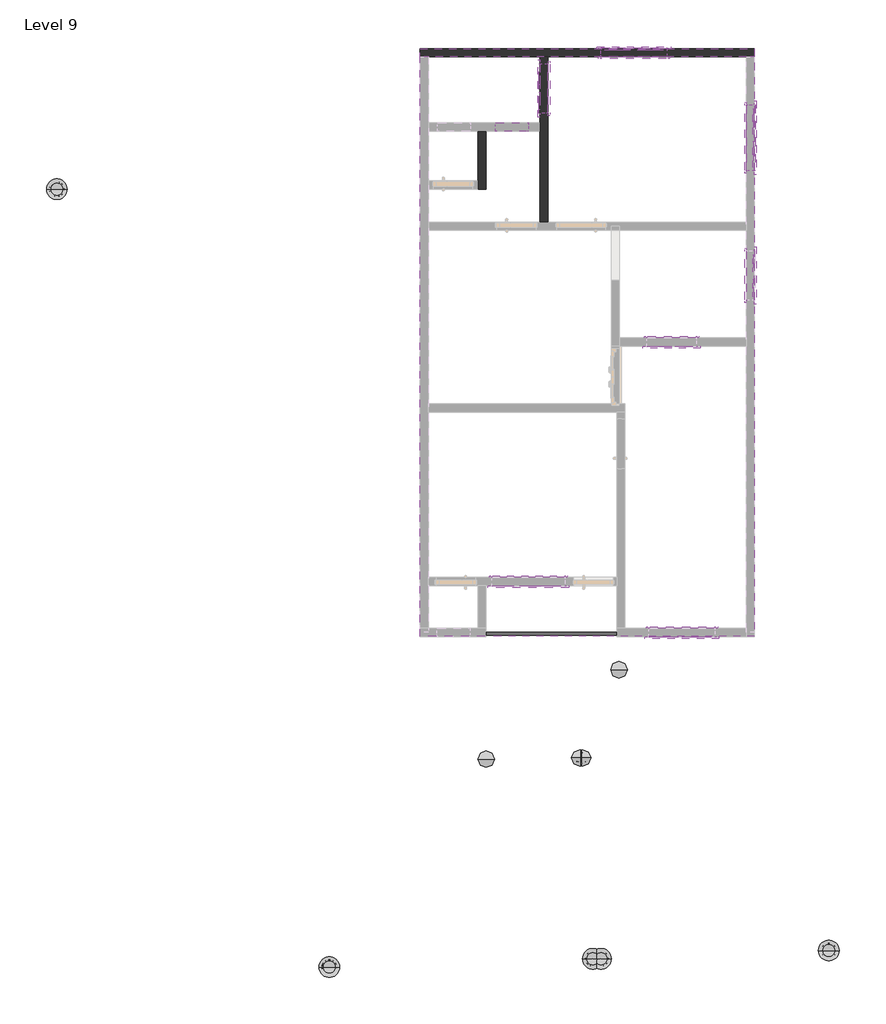
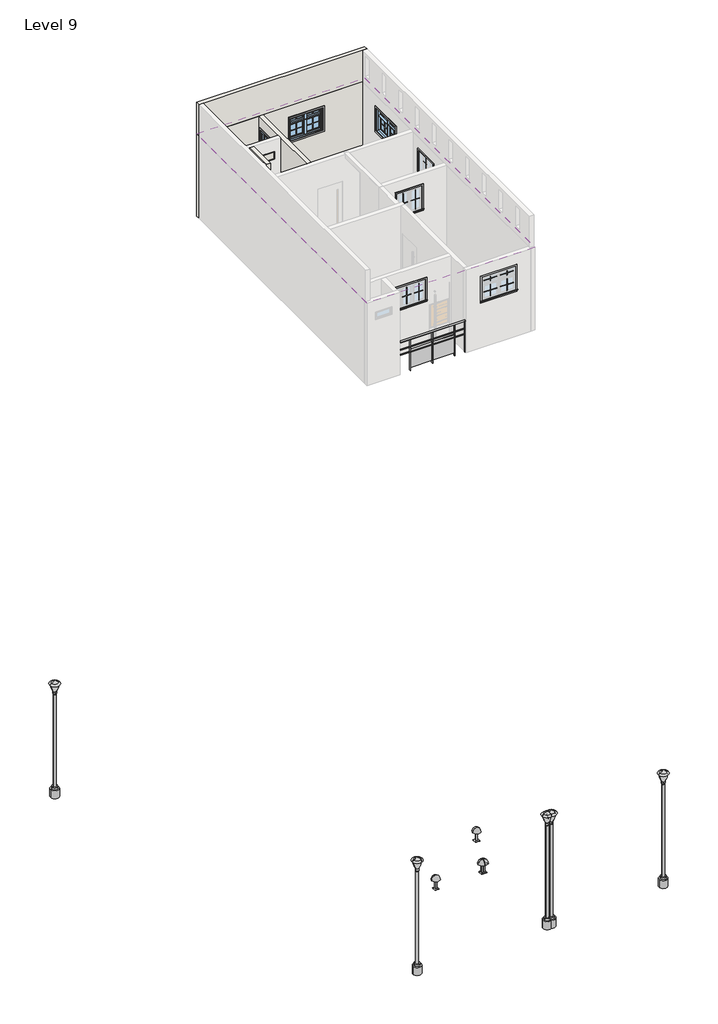
# One storey, part 2 of 2: 48 proxies, 10 light fixtures, 7 walls, 5 windows, 1 covering, 1 railing.
# Revit data of these elements (continued)
# Element 54 (IfcLightFixture, "M_Street Light - Antique : 400W Halogen - 120V")
#   Mark = "28"
#   Phase Created = New Construction
#   Materials on its faces: "Steel, Paint Finish, Dark Gray, Matte", "Glass, Frosted"
# Element 55 (IfcLightFixture, "M_Table Lamp - Hemispheric : 60W - 120V")
#   Mark = "8"
#   Phase Created = New Construction
#   Materials on its faces: "Steel, Chrome Plated", "Birch", "Plastic, Lamp Shade"
# Element 56 (IfcLightFixture, "M_Table Lamp - Hemispheric : 60W - 120V")
#   Mark = "9"
#   Phase Created = New Construction
#   Materials on its faces: "Steel, Chrome Plated", "Birch", "Plastic, Lamp Shade"
# Element 57 (IfcLightFixture, "M_Table Lamp - Hemispheric : 60W - 120V")
#   Mark = "10"
#   Phase Created = New Construction
#   Materials on its faces: "Steel, Chrome Plated", "Birch", "Plastic, Lamp Shade"
# Element 58 (IfcLightFixture, "M_Table Lamp - Hemispheric : 60W - 120V")
#   Mark = "11"
#   Phase Created = New Construction
#   Materials on its faces: "Steel, Chrome Plated", "Birch", "Plastic, Lamp Shade"
# Element 59 (IfcLightFixture, "M_Table Lamp - Hemispheric : 60W - 120V")
#   Mark = "13"
#   Phase Created = New Construction
#   Materials on its faces: "Steel, Chrome Plated", "Birch", "Plastic, Lamp Shade"
# Element 60 (IfcRailing, "Glass Panel - Bottom Fill")
#   Phase Created = New Construction
#   Materials on its faces: "Glass"
# Element 61 (IfcWall, "Generic - 6\"")
#   Top Offset = 0' - 0"
#   Base Offset = 0' - 0"
#   Unconnected Height = 10' - 6"
#   wall height = 10' - 6"
#   Phase Created = New Construction
#   Base Constraint = Level 9
#   Materials on its faces: "Default Wall", "Parking Stripe"
# Elements 62, 63, 64, 65, 66 (IfcWall, "Generic - 6\"")
#   Top Offset = 0' - 0"
#   Base Offset = 0' - 0"
#   Unconnected Height = 10' - 6"
#   wall height = 10' - 6"
#   Phase Created = New Construction
#   Base Constraint = Level 9
#   Materials on its faces: "Default Wall"
# Element 67 (IfcWall, "Generic - 6\"")
#   built-in parameter 1001111 = 10' - 6"
#   Top Offset = 0' - 0"
#   Base Offset = 10' - 6"
#   Unconnected Height = 4' - 0"
#   wall height = 4' - 0"
#   Phase Created = New Construction
#   Base Constraint = Level 9
#   Materials on its faces: "WALL", "Default Wall"
# Element 68 (IfcWindow, "Fixed : 2'")
#   Mark = "160"
#   Phase Created = New Construction
#   Materials on its faces: "Sash", "Glass"
# Element 69 (IfcWindow, "M_Window-Casement-Double : 3'")
#   Mark = "156"
#   Window Inset = 0' - 0"
#   Interior Wall Closure = 0' - 2.15551"
#   Frame Extension = 0' - 0 1/4"
#   Exterior Wall Closure = 0' - 1.25197"
#   Interior Trim Visibility = yes
#   Exterior Trim Visibility = yes
#   Phase Created = New Construction
#   Materials on its faces: "Wood - Stained", "Glass", "Clad - White"
# Element 70 (IfcWindow, "M_Window-Casement-Double : 3'")
#   Mark = "166"
#   Window Inset = 0' - 0"
#   Interior Wall Closure = 0' - 2.15551"
#   Frame Extension = 0' - 0 1/4"
#   Exterior Wall Closure = 0' - 1.25197"
#   Interior Trim Visibility = yes
#   Exterior Trim Visibility = yes
#   Phase Created = New Construction
#   Materials on its faces: "Wood - Stained", "Glass", "Clad - White"
# Element 71 (IfcWindow, "M_Window-Casement-Double-Awning-Double : 4'")
#   Mark = "151"
#   Window Inset = 0' - 0"
#   Interior Wall Closure = 0' - 2.15551"
#   Frame Extension = 0' - 0 1/4"
#   Exterior Wall Closure = 0' - 1.25197"
#   Interior Trim Visibility = yes
#   Exterior Trim Visibility = yes
#   Phase Created = New Construction
#   Materials on its faces: "Wood - Stained", "Glass", "Clad - White"
# Element 72 (IfcWindow, "M_Window-Casement-Double-Awning-Double : 4'")
#   Mark = "152"
#   Window Inset = 0' - 0"
#   Interior Wall Closure = 0' - 2.15551"
#   Frame Extension = 0' - 0 1/4"
#   Exterior Wall Closure = 0' - 1.25197"
#   Interior Trim Visibility = yes
#   Exterior Trim Visibility = yes
#   Phase Created = New Construction
#   Materials on its faces: "Wood - Stained", "Glass", "Clad - White"
# Materials
#   "Default": colour RGB 80 80 80, transparency 0
#   "Acoustic Ceiling Tile 24 x 48": class "Generic", colour RGB 180 179 177, transparency 0, Description = "Acoustic Ceiling Tile 24 x 48", Cost = 0
#   "Glass, Frosted": class "Glass", colour RGB 250 244 225, transparency 0.55, Description = "physical material", Cost = 0
#   "Steel, Paint Finish, Dark Gray, Matte": class "Metal", colour RGB 98 98 98, transparency 0, Description = "Steel, paint finish, dark gray, matte", Cost = 0
#   "Steel, Chrome Plated": class "Metal", colour RGB 244 244 244, transparency 0, Description = "Chromiuim plated steel", Cost = 0
#   "Plastic, Lamp Shade": class "Glass", colour RGB 250 244 225, transparency 0.58, Description = "physical material", Cost = 0
#   "Birch": class "Wood", colour RGB 224 178 126, transparency 0, Description = "Betula Alleghaniensis", Cost = 0
#   "Glass": class "Glass", colour RGB 218 227 224, transparency 0.85, Description = "Soda Lime Glass", Cost = 0
#   "Sash": class "Wood", colour RGB 136 99 55, transparency 0
#   "Wood - Stained": class "Wood", colour RGB 227 170 128, transparency 0, Cost = 0
#   "Clad - White": class "Wood", colour RGB 242 242 238, transparency 0, Cost = 0
#   "TILES 1": class "Generic", colour RGB 120 120 120, transparency 0, Cost = 0
#   "Default Wall": colour RGB 80 80 80, transparency 0
#   "Parking Stripe": class "Paint", colour RGB 226 219 42, transparency 0
#   "WALL": class "Generic", colour RGB 120 120 120, transparency 0, Cost = 0
